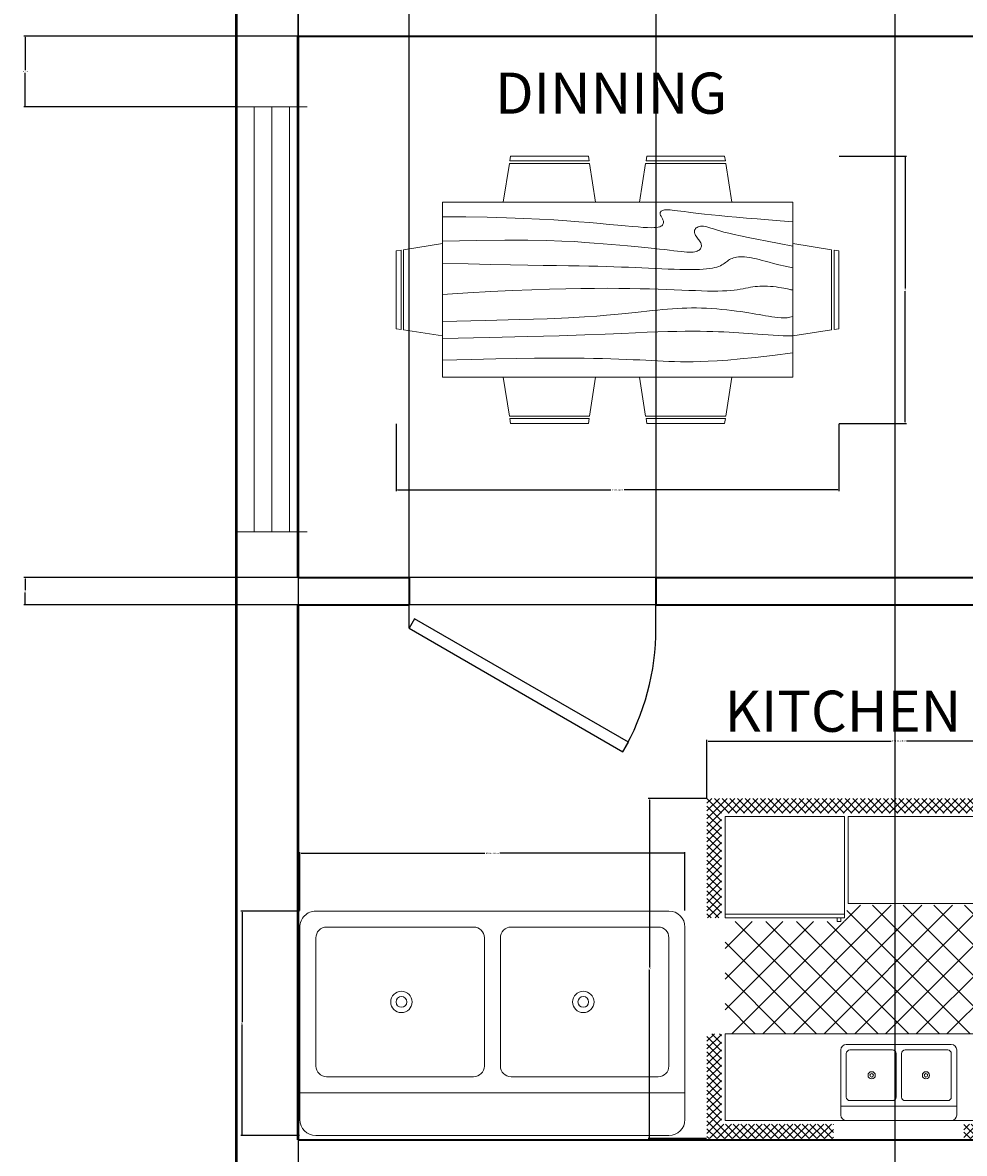
# Model space of a CAD drawing. Units: feet. Extents: x 3746 to 4170, y 1475 to 2148.
# Tile 2 of 5: x 3746 to 3884, y 1755 to 1920. Entities that reach past the tile are written whole.
import ezdxf

# ---------------------------------------------------------------- set-up
doc = ezdxf.new("R2010")
doc.units = ezdxf.units.FT
for name, color, linetype, lineweight in [('A-ANNO-DIMS', 2, 'Continuous', 18), ('A-AREA-IDEN', 7, 'Continuous', 25), ('A-FLOR-FIXT', 9, 'Continuous', 18), ('A-GLAZ', 91, 'Continuous', 18), ('DOOR', 135, 'Continuous', 25), ('FURNITURE', 43, 'Continuous', 18), ('INWER WALL', 30, 'Continuous', 35), ('OUTER WALL', 31, 'Continuous', 50)]:
    doc.layers.add(name, color=color, linetype=linetype, lineweight=lineweight)
doc.styles.get("Standard").update_dxf_attribs({"font": 'arial.ttf'})
doc.dimstyles.get("Standard").update_dxf_attribs({"dimtxt": 0.18, "dimasz": 0.18, "dimexe": 0.18, "dimexo": 0.0625, "dimgap": 0.09, "dimtad": 0, "dimtih": 1, "dimtoh": 1, "dimdec": 4, "dimzin": 0, "dimdsep": 46, "dimtxsty": 'Standard', "dimcen": 0.09, "dimadec": 0, "dimazin": 0, "dimtfac": 1, "dimtdec": 4, "dimtofl": 0, "dimtmove": 0, "dimatfit": 3, "dimfxl": 1, "dimtolj": 1, "dimtzin": 0, "dimarcsym": 0})

# ---------------------------------------------------------------- blocks, each defined once
blk = doc.blocks.new('*U3')
for p, q in [((0, 0), (0, 6)), ((40, 0), (40, 6))]:
    blk.add_line(p, q)
blk.add_lwpolyline([(0, 0), (34.64, -20), (35.52, -18.48), (0.87, 1.52)], close=True)
blk.add_arc((0, 0), 40, 330, 0)
blk = doc.blocks.new('Dining Set - 36 x 72 in.')
for p, q in [((-22.2343, 26.00059), (-23.4847, 17.99762)), ((-22.2304, 26), (-5.7608, 26)), ((-22, 27.5), (-22.1562, 26.50042)), ((-5.8416, 26.5), (-22.1534, 26.5)), ((-22, 27.5), (-6, 27.5)), ((-5.8437, 26.49966), (-6, 27.5)), ((-4.5152, 17.99762), (-5.7655, 25.99926)), ((5.7657, 26.00059), (4.5153, 17.99762)), ((5.7696, 26), (22.2392, 26)), ((6, 27.5), (5.8438, 26.50042)), ((22.1584, 26.5), (5.8466, 26.5)), ((6, 27.5), (22, 27.5)), ((22.1563, 26.49966), (22, 27.5)), ((23.4848, 17.99762), (22.2345, 25.99926)), ((36, 18), (-36, 18)), ((-36, 18), (-36, -18)), ((36, -18), (36, 18)), ((-44.0006, 8.23428), (-35.9976, 9.48474)), ((44.0006, 8.23428), (35.9976, 9.48474)), ((-45.5, 8), (-44.5004, 8.15617)), ((-45.5, 8), (-45.5, -8)), ((-44.5, -8.15843), (-44.5, 8.15338)), ((-44, 8.23041), (-44, -8.23915)), ((44, 8.23041), (44, -8.23915)), ((44.5, -8.15843), (44.5, 8.15338)), ((45.5, 8), (44.5005, 8.15617)), ((45.5, 8), (45.5, -8)), ((-44.4997, -8.15631), (-45.5, -8)), ((-35.9976, -9.48476), (-43.9993, -8.2345)), ((35.9976, -9.48476), (43.9993, -8.2345)), ((44.4997, -8.15631), (45.5, -8)), ((-36, -18), (36, -18)), ((-22.2343, -26.0006), (-23.4847, -17.99762)), ((-4.5152, -17.99762), (-5.7655, -25.99928)), ((5.7657, -26.0006), (4.5153, -17.99762)), ((23.4848, -17.99762), (22.2345, -25.99928)), ((-22.2304, -26), (-5.7608, -26)), ((-22, -27.5), (-22.1562, -26.50044)), ((-5.8416, -26.5), (-22.1534, -26.5)), ((-22, -27.5), (-6, -27.5)), ((-5.8437, -26.49967), (-6, -27.5)), ((5.7696, -26), (22.2392, -26)), ((6, -27.5), (5.8438, -26.50044)), ((22.1584, -26.5), (5.8466, -26.5)), ((6, -27.5), (22, -27.5)), ((22.1563, -26.49967), (22, -27.5))]:
    blk.add_line(p, q)
for points in [[(-36, 15), (-31.1772, 14.97754), (-26.8079, 14.91406), (-22.8538, 14.81543), (-19.276, 14.6875), (-16.0362, 14.53613), (-13.0957, 14.36718), (-10.4159, 14.18652), (-7.9583, 14), (-5.6904, 13.81315), (-3.6035, 13.63021), (-1.6954, 13.45508), (0.0365, 13.29166), (1.5945, 13.14388), (2.9811, 13.01562), (4.1988, 12.9108), (5.25, 12.83333), (6.1393, 12.78613), (6.8802, 12.76823), (7.4883, 12.77767), (7.9792, 12.8125), (8.3685, 12.87077), (8.6719, 12.95052), (8.9049, 13.0498), (9.0833, 13.16666), (9.2205, 13.29899), (9.3216, 13.44401), (9.3895, 13.59879), (9.4271, 13.76041), (9.4373, 13.92594), (9.4232, 14.09245), (9.3875, 14.257), (9.3333, 14.41666), (9.2638, 14.56917), (9.1836, 14.71484), (9.0975, 14.85465), (9.0104, 14.98958), (8.9272, 15.1206), (8.8529, 15.2487), (8.7922, 15.37483), (8.75, 15.5), (8.7305, 15.62467), (8.7344, 15.74739), (8.7617, 15.86621), (8.8125, 15.97916), (8.8867, 16.08431), (8.9844, 16.17968), (9.1055, 16.26334), (9.25, 16.33333), (9.4189, 16.38802), (9.6172, 16.42708), (9.8506, 16.45052), (10.125, 16.45833), (10.4463, 16.45052), (10.8203, 16.42708), (11.2529, 16.38802), (11.75, 16.33333), (12.3184, 16.26318), (12.9694, 16.17838), (13.7151, 16.07991), (14.5677, 15.96875), (15.5395, 15.84586), (16.6426, 15.71224), (17.8893, 15.56884), (19.2917, 15.41666), (20.859, 15.25667), (22.5879, 15.08984), (24.4721, 14.91715), (26.5052, 14.73958), (28.6809, 14.5581), (30.9929, 14.3737), (33.4347, 14.18733), (36, 14)], [(-36, 10), (-28.9766, 10.14274), (-23.1725, 10.20442), (-18.4241, 10.19775), (-14.5677, 10.13541), (-11.4399, 10.03011), (-8.877, 9.89453), (-6.7154, 9.74137), (-4.7917, 9.58333), (-2.9698, 9.43082), (-1.2246, 9.28515), (0.4415, 9.14534), (2.026, 9.01041), (3.5266, 8.87939), (4.9408, 8.7513), (6.266, 8.62516), (7.5, 8.5), (8.6411, 8.37549), (9.6914, 8.2539), (10.6538, 8.13818), (11.5312, 8.03125), (12.3267, 7.93603), (13.043, 7.85547), (13.6831, 7.79248), (14.25, 7.75), (14.7471, 7.7303), (15.1797, 7.73307), (15.5537, 7.75732), (15.875, 7.80208), (16.1494, 7.86637), (16.3828, 7.94922), (16.5811, 8.04964), (16.75, 8.16666), (16.8944, 8.29915), (17.0143, 8.44531), (17.1089, 8.60319), (17.1771, 8.77083), (17.218, 8.94629), (17.2305, 9.1276), (17.2137, 9.31282), (17.1667, 9.5), (17.0895, 9.6875), (16.987, 9.875), (16.8649, 10.0625), (16.7292, 10.25), (16.5856, 10.4375), (16.4401, 10.625), (16.2985, 10.8125), (16.1667, 11), (16.05, 11.18733), (15.9518, 11.3737), (15.8752, 11.5581), (15.8229, 11.73958), (15.798, 11.91715), (15.8034, 12.08984), (15.842, 12.25667), (15.9167, 12.41666), (16.0295, 12.56836), (16.1784, 12.70833), (16.3605, 12.83268), (16.5729, 12.9375), (16.8127, 13.01888), (17.0768, 13.07291), (17.3625, 13.0957), (17.6667, 13.08333), (17.9894, 13.03312), (18.3418, 12.94726), (18.7382, 12.82918), (19.1927, 12.68229), (19.7195, 12.51001), (20.3327, 12.31575), (21.0465, 12.10294), (21.875, 11.875), (22.8357, 11.63354), (23.959, 11.37304), (25.2786, 11.08618), (26.8282, 10.76562), (28.6414, 10.40405), (30.752, 9.99414), (33.1936, 9.52856), (36, 9)], [(-36, 5.5), (-30.7157, 5.3348), (-26.069, 5.20963), (-21.9946, 5.11767), (-18.4271, 5.05208), (-15.3009, 5.00602), (-12.5508, 4.97265), (-10.1112, 4.94515), (-7.9167, 4.91666), (-5.909, 4.88167), (-4.0586, 4.83984), (-2.3429, 4.79215), (-0.7396, 4.73958), (0.7739, 4.6831), (2.22, 4.6237), (3.6213, 4.56233), (5, 4.5), (6.373, 4.43782), (7.7344, 4.3776), (9.0723, 4.32129), (10.375, 4.27083), (11.6309, 4.22819), (12.8281, 4.19531), (13.9551, 4.17415), (15, 4.16666), (15.954, 4.17448), (16.819, 4.19791), (17.6001, 4.23698), (18.3021, 4.29166), (18.9299, 4.36198), (19.4883, 4.44791), (19.9823, 4.54948), (20.4167, 4.66666), (20.7969, 4.79899), (21.1302, 4.94401), (21.4245, 5.09879), (21.6875, 5.26041), (21.9271, 5.42594), (22.1511, 5.59245), (22.3672, 5.757), (22.5834, 5.91666), (22.8065, 6.06868), (23.0404, 6.21093), (23.2879, 6.34147), (23.5521, 6.45833), (23.8358, 6.55957), (24.142, 6.64323), (24.4735, 6.70735), (24.8334, 6.75), (25.2235, 6.76969), (25.642, 6.76692), (26.0858, 6.74267), (26.5521, 6.69791), (27.0379, 6.63362), (27.5404, 6.55078), (28.0565, 6.45036), (28.5834, 6.33333), (29.1242, 6.19987), (29.7071, 6.04687), (30.3661, 5.87044), (31.1354, 5.66666), (32.0493, 5.43164), (33.142, 5.16146), (34.4475, 4.85221), (36, 4.5)], [(-36, -1), (-30.7915, -0.6591), (-26.0195, -0.38216), (-21.6519, -0.16284), (-17.6563, 0.00521), (-14.0005, 0.12833), (-10.6523, 0.21289), (-7.5796, 0.26522), (-4.75, 0.29166), (-2.134, 0.29793), (0.2878, 0.28711), (2.5317, 0.26163), (4.6146, 0.22396), (6.5529, 0.17651), (8.3633, 0.12174), (10.0623, 0.06209), (11.6667, 0), (13.1899, -0.06201), (14.6341, -0.1211), (15.9982, -0.17432), (17.2813, -0.21875), (18.4823, -0.25147), (19.6003, -0.26953), (20.6343, -0.27002), (21.5834, -0.25), (22.4481, -0.20768), (23.2357, -0.14584), (23.9549, -0.06836), (24.6146, 0.02083), (25.2235, 0.11784), (25.7904, 0.21875), (26.3241, 0.31966), (26.8334, 0.41666), (27.3265, 0.50618), (27.8099, 0.58593), (28.2894, 0.65397), (28.7709, 0.70833), (29.2601, 0.74707), (29.763, 0.76823), (30.2855, 0.76985), (30.8334, 0.75), (31.4088, 0.70784), (31.9994, 0.64713), (32.589, 0.57275), (33.1615, 0.48958), (33.7008, 0.4025), (34.1908, 0.3164), (34.6153, 0.23616), (34.9584, 0.16666), (35.2099, 0.11165), (35.3848, 0.07031), (35.504, 0.04069), (35.5886, 0.02083), (35.6594, 0.00879), (35.7377, 0.0026), (35.8442, 0.00032), (36, 0)], [(-36, -6.5), (-27.1843, -6.31267), (-20.084, -6.1263), (-14.469, -5.9419), (-10.1094, -5.76042), (-6.7752, -5.58285), (-4.2363, -5.41016), (-2.2629, -5.24333), (-0.625, -5.08334), (0.8708, -4.93099), (2.2715, -4.78646), (3.5872, -4.64974), (4.8281, -4.52084), (6.0046, -4.39974), (7.127, -4.28646), (8.2053, -4.18099), (9.25, -4.08334), (10.2705, -3.99382), (11.2734, -3.91407), (12.2647, -3.84603), (13.25, -3.79167), (14.2354, -3.75293), (15.2266, -3.73177), (16.2295, -3.73015), (17.25, -3.75), (18.2912, -3.79248), (19.3451, -3.85547), (20.4009, -3.93604), (21.4479, -4.03125), (22.4754, -4.13819), (23.4727, -4.25391), (24.4289, -4.37549), (25.3334, -4.5), (26.1785, -4.62492), (26.9694, -4.74935), (27.7145, -4.87281), (28.4219, -4.99479), (29.1, -5.11483), (29.7572, -5.23242), (30.4016, -5.34709), (31.0417, -5.45834), (31.6837, -5.56437), (32.3262, -5.65821), (32.9658, -5.73153), (33.599, -5.77604), (34.2224, -5.78345), (34.8327, -5.74545), (35.4264, -5.65373), (36, -5.5)], [(-36, -10), (-26.4022, -9.81299), (-18.4675, -9.62891), (-11.9839, -9.45069), (-6.7396, -9.28125), (-2.5226, -9.12354), (0.8789, -8.98047), (3.6769, -8.85498), (6.0833, -8.75), (8.2767, -8.66765), (10.3021, -8.60677), (12.1712, -8.56543), (13.8958, -8.54167), (15.4876, -8.53353), (16.9583, -8.53907), (18.3197, -8.55632), (19.5834, -8.58334), (20.7616, -8.61841), (21.8685, -8.66081), (22.9188, -8.71004), (23.9271, -8.76563), (24.9081, -8.82707), (25.8763, -8.89388), (26.8465, -8.96558), (27.8334, -9.04167), (28.8474, -9.12118), (29.8828, -9.20117), (30.93, -9.27824), (31.9792, -9.34896), (33.0205, -9.40991), (34.0443, -9.45768), (35.0407, -9.48885), (36, -9.5)], [(-36, -14.5), (-30.0881, -14.33513), (-25.0332, -14.21224), (-20.7312, -14.12647), (-17.0781, -14.07292), (-13.97, -14.04671), (-11.3027, -14.04297), (-8.9724, -14.05681), (-6.875, -14.08334), (-4.9224, -14.11833), (-3.0905, -14.16016), (-1.3709, -14.20785), (0.2448, -14.26042), (1.7647, -14.3169), (3.1973, -14.3763), (4.5507, -14.43767), (5.8333, -14.5), (7.0554, -14.5621), (8.235, -14.62175), (9.3922, -14.67652), (10.5469, -14.72396), (11.7192, -14.76164), (12.929, -14.78711), (14.1965, -14.79794), (15.5417, -14.79167), (16.9933, -14.76424), (18.6152, -14.70508), (20.4804, -14.60197), (22.6615, -14.44271), (25.2312, -14.21509), (28.2624, -13.9069), (31.8277, -13.50594), (36, -13)]]:
    blk.add_lwpolyline(points)
blk = doc.blocks.new('Kitchen Layout - 7 x 8 ft')
for p, q in [((-5, 81.32), (2.68, 89)), ((-5, 83.44), (0.56, 89)), ((-5, 85.56), (-1.56, 89)), ((-5, 87.68), (-3.68, 89)), ((-1, 84.97), (-5, 88.97)), ((1.09, 85), (-2.91, 89)), ((3.21, 85), (-0.79, 89)), ((0.81, 85), (4.81, 89)), ((5.34, 85), (1.34, 89)), ((2.93, 85), (6.93, 89)), ((7.46, 85), (3.46, 89)), ((5.05, 85), (9.05, 89)), ((9.58, 85), (5.58, 89)), ((7.17, 85), (11.17, 89)), ((11.7, 85), (7.7, 89)), ((9.29, 85), (13.29, 89)), ((13.82, 85), (9.82, 89)), ((11.41, 85), (15.41, 89)), ((15.94, 85), (11.94, 89)), ((13.53, 85), (17.53, 89)), ((18.06, 85), (14.06, 89)), ((15.65, 85), (19.65, 89)), ((20.18, 85), (16.18, 89)), ((17.78, 85), (21.78, 89)), ((22.31, 85), (18.31, 89)), ((19.9, 85), (23.9, 89)), ((24.43, 85), (20.43, 89)), ((22.02, 85), (26.02, 89)), ((26.55, 85), (22.55, 89)), ((24.14, 85), (28.14, 89)), ((28.67, 85), (24.67, 89)), ((26.26, 85), (30.26, 89)), ((30.79, 85), (26.79, 89)), ((28.38, 85), (32.38, 89)), ((32.91, 85), (28.91, 89)), ((30.5, 85), (34.5, 89)), ((35.03, 85), (31.03, 89)), ((32.63, 85), (36.63, 89)), ((37.16, 85), (33.16, 89)), ((34.75, 85), (38.75, 89)), ((39.28, 85), (35.28, 89)), ((36.87, 85), (40.87, 89)), ((41.4, 85), (37.4, 89)), ((38.99, 85), (42.99, 89)), ((43.52, 85), (39.52, 89)), ((41.11, 85), (45.11, 89)), ((45.64, 85), (41.64, 89)), ((43.23, 85), (47.23, 89)), ((47.76, 85), (43.76, 89)), ((45.35, 85), (49.35, 89)), ((49.88, 85), (45.88, 89)), ((47.47, 85), (51.47, 89)), ((52, 85), (48, 89)), ((49.6, 85), (53.6, 89)), ((54.13, 85), (50.13, 89)), ((51.72, 85), (55.72, 89)), ((56.25, 85), (52.25, 89)), ((53.84, 85), (57.84, 89)), ((58.37, 85), (54.37, 89)), ((55.96, 85), (59.96, 89)), ((60.49, 85), (56.49, 89)), ((58.08, 85), (62.08, 89)), ((62.61, 85), (58.61, 89)), ((60.2, 85), (64.2, 89)), ((64.73, 85), (60.73, 89)), ((62.32, 85), (66.32, 89)), ((66.85, 85), (62.85, 89)), ((64.45, 85), (68.45, 89)), ((68.97, 85), (64.97, 89)), ((66.57, 85), (70.57, 89)), ((71.1, 85), (67.1, 89)), ((68.69, 85), (72.69, 89)), ((73.22, 85), (69.22, 89)), ((70.81, 85), (74.81, 89)), ((75.34, 85), (71.34, 89)), ((72.93, 85), (76.93, 89)), ((77.46, 85), (73.46, 89)), ((75.05, 85), (79.05, 89)), ((79.58, 85), (75.58, 89)), ((77.17, 85), (81.17, 89)), ((81.7, 85), (77.7, 89)), ((79.29, 85), (83.29, 89)), ((83.82, 85), (79.82, 89)), ((81.42, 85), (85.42, 89)), ((85.95, 85), (81.95, 89)), ((83.54, 85), (87.54, 89)), ((88.07, 85), (84.07, 89)), ((85.66, 85), (89.66, 89)), ((90.19, 85), (86.19, 89)), ((87.78, 85), (91.78, 89)), ((92.31, 85), (88.31, 89)), ((89.9, 85), (93.9, 89)), ((94.43, 85), (90.43, 89)), ((92.02, 85), (96.02, 89)), ((96.55, 85), (92.55, 89)), ((94.14, 85), (98.14, 89)), ((101, 82.67), (94.67, 89)), ((96.27, 85), (100.27, 89)), ((101, 84.79), (96.79, 89)), ((97, 83.61), (101, 87.61)), ((101, 86.92), (98.92, 89)), ((-1, 82.85), (-5, 86.85)), ((-1, 80.73), (-5, 84.73)), ((97, 81.49), (101, 85.49)), ((101, 80.55), (97, 84.55)), ((-5, 79.19), (-1, 83.19)), ((-1, 78.61), (-5, 82.61)), ((34, 84), (96, 84)), ((34, 60), (34, 84)), ((96, 84), (96, 60)), ((97, 79.37), (101, 83.37)), ((101, 78.43), (97, 82.43)), ((-5, 77.07), (-1, 81.07)), ((-1, 76.49), (-5, 80.49)), ((-5, 74.95), (-1, 78.95)), ((-1, 74.36), (-5, 78.36)), ((74, 81), (95, 81)), ((97, 77.25), (101, 81.25)), ((101, 76.31), (97, 80.31)), ((97, 75.13), (101, 79.13)), ((101, 74.19), (97, 78.19)), ((-5, 72.83), (-1, 76.83)), ((-1, 72.24), (-5, 76.24)), ((97, 73.01), (101, 77.01)), ((101, 72.07), (97, 76.07)), ((-5, 70.71), (-1, 74.71)), ((-1, 70.12), (-5, 74.12)), ((-5, 68.59), (-1, 72.59)), ((-1, 68), (-5, 72)), ((97, 70.89), (101, 74.89)), ((101, 69.95), (97, 73.95)), ((97, 68.76), (101, 72.76)), ((-5, 66.47), (-1, 70.47)), ((-1, 65.88), (-5, 69.88)), ((101, 67.82), (97, 71.82)), ((97, 66.64), (101, 70.64)), ((101, 65.7), (97, 69.7)), ((-5, 64.35), (-1, 68.35)), ((-1, 63.76), (-5, 67.76)), ((-5, 62.22), (-1, 66.22)), ((-1, 61.64), (-5, 65.64)), ((97, 64.52), (101, 68.52)), ((101, 63.58), (97, 67.58)), ((97, 62.4), (101, 66.4)), ((-5, 60.1), (-1, 64.1)), ((-1, 59.52), (-5, 63.52)), ((101, 61.46), (97, 65.46)), ((97, 60.28), (101, 64.28)), ((100.34, 60), (97, 63.34)), ((-5, 57.98), (-1, 61.98)), ((-1, 57.39), (-5, 61.39)), ((-4.86, 56), (-1, 59.86)), ((10.4, 24), (45.9, 59.5)), ((18.88, 24), (54.38, 59.5)), ((27.37, 24), (62.87, 59.5)), ((33.03, 55.11), (37.41, 59.5)), ((96, 60), (34, 60)), ((35.85, 24), (71.35, 59.5)), ((76.2, 24), (40.7, 59.5)), ((84.68, 24), (49.18, 59.5)), ((93.17, 24), (57.67, 59.5)), ((96, 29.65), (66.15, 59.5)), ((80, 60), (80, 59)), ((82, 59), (82, 60)), ((87, 59), (87, 60)), ((89, 60), (89, 59)), ((98.22, 60), (97, 61.22)), ((98.84, 60), (101, 62.16)), ((100.96, 60), (101, 60.04)), ((-1.73, 56), (-5, 59.27)), ((-3.85, 56), (-5, 57.15)), ((-2.74, 56), (-1, 57.74)), ((0, 57), (33, 57)), ((67.71, 24), (33.68, 58.04)), ((44.34, 24), (77.84, 57.5)), ((52.82, 24), (86.32, 57.5)), ((61.31, 24), (96, 58.69)), ((96, 38.14), (76.64, 57.5)), ((96, 46.63), (85.13, 57.5)), ((96, 55.11), (93.57, 57.54)), ((0, 30.57), (24.43, 55)), ((0, 39.06), (15.94, 55)), ((0, 47.54), (7.46, 55)), ((1.91, 24), (32.91, 55)), ((33.77, 24), (2.77, 55)), ((42.26, 24), (11.26, 55)), ((50.74, 24), (19.74, 55)), ((59.23, 24), (28.23, 55)), ((31, 55), (31, 56)), ((32, 55), (31, 55)), ((32, 56), (32, 55)), ((69.79, 24), (96, 50.21)), ((25.29, 24), (0, 49.29)), ((16.8, 24), (0, 40.8)), ((78.28, 24), (96, 41.72)), ((8.32, 24), (0, 32.32)), ((86.76, 24), (96, 33.24)), ((-5, 21.92), (-2.92, 24)), ((-5, 19.8), (-1, 23.8)), ((-1, 19.21), (-5, 23.21)), ((-1, 21.33), (-3.67, 24)), ((-1, 23.45), (-1.55, 24)), ((0, 24), (96, 24)), ((0, 0), (0, 24)), ((95.25, 24), (96, 24.75)), ((96, 24), (96, 0)), ((97, 22.1), (98.9, 24)), ((97, 19.97), (101, 23.97)), ((101, 19.03), (97, 23.03)), ((101, 21.16), (98.16, 24)), ((101, 23.28), (100.28, 24)), ((-5, 17.68), (-1, 21.68)), ((-1, 17.09), (-5, 21.09)), ((-5, 15.55), (-1, 19.55)), ((-1, 14.97), (-5, 18.97)), ((97, 17.85), (101, 21.85)), ((101, 16.91), (97, 20.91)), ((97, 15.73), (101, 19.73)), ((101, 14.79), (97, 18.79)), ((-5, 13.43), (-1, 17.43)), ((-1, 12.85), (-5, 16.85)), ((47.25, 6.5), (47.25, 18.5)), ((48.75, 18.5), (48.75, 6.5)), ((97, 13.61), (101, 17.61)), ((101, 12.67), (97, 16.67)), ((-5, 11.31), (-1, 15.31)), ((-1, 10.73), (-5, 14.73)), ((-5, 9.19), (-1, 13.19)), ((-1, 8.6), (-5, 12.6)), ((97, 11.49), (101, 15.49)), ((101, 10.55), (97, 14.55)), ((97, 9.37), (101, 13.37)), ((-5, 7.07), (-1, 11.07)), ((-1, 6.48), (-5, 10.48)), ((101, 8.43), (97, 12.43)), ((97, 7.25), (101, 11.25)), ((101, 6.31), (97, 10.31)), ((-5, 4.95), (-1, 8.95)), ((-1, 4.36), (-5, 8.36)), ((-5, 2.83), (-1, 6.83)), ((97, 5.12), (101, 9.12)), ((101, 4.18), (97, 8.18)), ((97, 3), (101, 7)), ((-1, 2.24), (-5, 6.24)), ((-5, 0.71), (-1, 4.71)), ((-1, 0.12), (-5, 4.12)), ((64, 4), (32, 4)), ((101, 2.06), (97, 6.06)), ((97, 0.88), (101, 4.88)), ((101, -0.06), (97, 3.94)), ((-5, -1.42), (-1, 2.58)), ((2, -5), (-5, 2)), ((-5, -3.54), (-1, 0.46)), ((96, 0), (0, 0)), ((93.24, -5), (101, 2.76)), ((95.36, -5), (101, 0.64)), ((101, -2.18), (97, 1.82)), ((-0.12, -5), (-5, -0.12)), ((-2.25, -5), (-5, -2.25)), ((-4.34, -5), (-0.34, -1)), ((-2.22, -5), (1.78, -1)), ((-0.1, -5), (3.9, -1)), ((4.12, -5), (0.12, -1)), ((2.02, -5), (6.02, -1)), ((6.24, -5), (2.24, -1)), ((4.14, -5), (8.14, -1)), ((8.36, -5), (4.36, -1)), ((6.27, -5), (10.27, -1)), ((10.48, -5), (6.48, -1)), ((8.39, -5), (12.39, -1)), ((12.6, -5), (8.6, -1)), ((10.51, -5), (14.51, -1)), ((14.73, -5), (10.73, -1)), ((12.63, -5), (16.63, -1)), ((16.85, -5), (12.85, -1)), ((14.75, -5), (18.75, -1)), ((18.97, -5), (14.97, -1)), ((16.87, -5), (20.87, -1)), ((21.09, -5), (17.09, -1)), ((18.99, -5), (22.99, -1)), ((23.21, -5), (19.21, -1)), ((21.11, -5), (25.11, -1)), ((25.33, -5), (21.33, -1)), ((23.24, -5), (27.24, -1)), ((27.45, -5), (23.45, -1)), ((25.36, -5), (29.36, -1)), ((29.57, -5), (25.57, -1)), ((27.48, -5), (30, -2.48)), ((30, -3.3), (27.7, -1)), ((30, -1.18), (29.82, -1)), ((66, -2.54), (67.54, -1)), ((66, -4.66), (69.66, -1)), ((69.88, -5), (66, -1.12)), ((67.78, -5), (71.78, -1)), ((72, -5), (68, -1)), ((69.9, -5), (73.9, -1)), ((74.12, -5), (70.12, -1)), ((72.03, -5), (76.03, -1)), ((76.24, -5), (72.24, -1)), ((74.15, -5), (78.15, -1)), ((78.36, -5), (74.36, -1)), ((76.27, -5), (80.27, -1)), ((80.49, -5), (76.49, -1)), ((78.39, -5), (82.39, -1)), ((82.61, -5), (78.61, -1)), ((80.51, -5), (84.51, -1)), ((84.73, -5), (80.73, -1)), ((82.63, -5), (86.63, -1)), ((86.85, -5), (82.85, -1)), ((84.75, -5), (88.75, -1)), ((88.97, -5), (84.97, -1)), ((86.88, -5), (90.88, -1)), ((91.09, -5), (87.09, -1)), ((89, -5), (93, -1)), ((93.21, -5), (89.21, -1)), ((91.12, -5), (95.12, -1)), ((95.34, -5), (91.34, -1)), ((97.46, -5), (93.46, -1)), ((99.58, -5), (95.58, -1)), ((101, -4.3), (97, -0.3)), ((97.48, -5), (101, -1.48)), ((-4.37, -5), (-5, -4.37)), ((29.6, -5), (30, -4.6)), ((67.76, -5), (66, -3.24)), ((99.6, -5), (101, -3.6))]:
    blk.add_line(p, q)
for points in [[(0, 56), (0, 84), (33, 84), (33, 56)], [(74, 60), (74, 84), (95, 84), (95, 60)], [(76, 58), (76, 59), (93, 59), (93, 58)]]:
    blk.add_lwpolyline(points, close=True)
for points in [[(32, 1.5), (32, 19.5)], [(33.5, 21), (62.5, 21)], [(34.5, 19.5), (46.25, 19.5)], [(49.75, 19.5), (61.5, 19.5)], [(64, 19.5), (64, 1.5)], [(33.5, 6.5), (33.5, 18.5)], [(62.5, 18.5), (62.5, 6.5)], [(46.25, 5.5), (34.5, 5.5)], [(61.5, 5.5), (49.75, 5.5)], [(62.5, 0), (33.5, 0)]]:
    blk.add_lwpolyline(points)
for centre, radius in [((80, 75), 4), ((80, 75), 3), ((80, 75), 2), ((80, 75), 1), ((89, 75), 3), ((89, 75), 2), ((89, 75), 1), ((80, 66), 3), ((89, 66), 4), ((89, 66), 3), ((80, 66), 2), ((80, 66), 1), ((89, 66), 2), ((89, 66), 1), ((40.5, 12.5), 1), ((40.5, 12.5), 0.5), ((55.5, 12.5), 1), ((55.5, 12.5), 0.5)]:
    blk.add_circle(centre, radius)
for centre, radius, start, end in [((33.5, 19.5), 1.5, 90, 180), ((34.5, 18.5), 1, 90, 180), ((46.25, 18.5), 1, 0, 90), ((49.75, 18.5), 1, 90, 180), ((61.5, 18.5), 1, 0, 90), ((62.5, 19.5), 1.5, 0, 90), ((34.5, 6.5), 1, 180, 270), ((46.25, 6.5), 1, 270, 0), ((49.75, 6.5), 1, 180, 270), ((61.5, 6.5), 1, 270, 0), ((33.5, 1.5), 1.5, 180, 270), ((62.5, 1.5), 1.5, 270, 0)]:
    blk.add_arc(centre, radius, start, end)
blk = doc.blocks.new('Sink-double - 36 in top')
for p, q in [((-18, -4), (18, -4)), ((-0.75, -18.5), (-0.75, -6.5)), ((0.75, -6.5), (0.75, -18.5))]:
    blk.add_line(p, q)
for points in [[(-16.5, 0), (16.5, 0)], [(-18, -19.5), (-18, -1.5)], [(18, -1.5), (18, -19.5)], [(-15.5, -5.5), (-1.75, -5.5)], [(1.75, -5.5), (15.5, -5.5)], [(-16.5, -18.5), (-16.5, -6.5)], [(16.5, -6.5), (16.5, -18.5)], [(-1.75, -19.5), (-15.5, -19.5)], [(15.5, -19.5), (1.75, -19.5)], [(16.5, -21), (-16.5, -21)]]:
    blk.add_lwpolyline(points)
for centre, radius in [((-8.5, -12.5), 1), ((8.5, -12.5), 1), ((-8.5, -12.5), 0.5), ((8.5, -12.5), 0.5)]:
    blk.add_circle(centre, radius)
for centre, radius, start, end in [((-16.5, -1.5), 1.5, 90, 180), ((16.5, -1.5), 1.5, 0, 90), ((-15.5, -6.5), 1, 90, 180), ((-1.75, -6.5), 1, 0, 90), ((1.75, -6.5), 1, 90, 180), ((15.5, -6.5), 1, 0, 90), ((-15.5, -18.5), 1, 180, 270), ((-1.75, -18.5), 1, 270, 0), ((1.75, -18.5), 1, 180, 270), ((15.5, -18.5), 1, 270, 0), ((-16.5, -19.5), 1.5, 180, 270), ((16.5, -19.5), 1.5, 270, 0)]:
    blk.add_arc(centre, radius, start, end)
blk = doc.blocks.new('Window - Wood Frame 36 in. Wide plan')
for p, q in [((0, 6), (0, 0)), ((36, 6), (36, 0)), ((0, 4.5), (36, 4.5)), ((0, 3), (36, 3)), ((0, 1.5), (36, 1.5))]:
    blk.add_line(p, q)
blk = doc.blocks.new('*D47')
at = {"layer": 'A-ANNO-DIMS', "color": 0, "lineweight": -2, "transparency": 16777216}
for p, q in [((3800.73, 1861.79), (3800.73, 1851.99)), ((3865.28, 1861.79), (3865.28, 1851.99)), ((3800.91, 1852.17), (3832.04, 1852.17)), ((3865.1, 1852.17), (3833.97, 1852.17))]:
    blk.add_line(p, q, dxfattribs=at)
at = {"layer": 'A-ANNO-DIMS', "color": 0, "transparency": 16777216}
for points in [[(3800.91, 1852.2), (3800.91, 1852.14), (3800.73, 1852.17)], [(3865.1, 1852.2), (3865.1, 1852.14), (3865.28, 1852.17)]]:
    blk.add_solid(points, dxfattribs=at)
at = {"layer": 'Defpoints', "color": 0, "transparency": 16777216}
for p in [(3800.73, 1861.86), (3865.28, 1861.86), (3865.28, 1852.17)]:
    blk.add_point(p, dxfattribs=at)
at = {"layer": 'A-ANNO-DIMS', "color": 0, "transparency": 16777216, "insert": (3833, 1852.17), "char_height": 0.18, "attachment_point": 5}
blk.add_mtext('\\A1;DINING SET 65', dxfattribs=at)
blk = doc.blocks.new('*D48')
at = {"layer": 'A-ANNO-DIMS', "color": 0, "lineweight": -2, "transparency": 16777216}
for p, q in [((3865.34, 1900.87), (3875.14, 1900.87)), ((3874.96, 1900.69), (3874.96, 1881.55)), ((3874.96, 1862.04), (3874.96, 1881.18)), ((3865.34, 1861.86), (3875.14, 1861.86))]:
    blk.add_line(p, q, dxfattribs=at)
at = {"layer": 'A-ANNO-DIMS', "color": 0, "transparency": 16777216}
for points in [[(3874.93, 1900.69), (3874.99, 1900.69), (3874.96, 1900.87)], [(3874.93, 1862.04), (3874.99, 1862.04), (3874.96, 1861.86)]]:
    blk.add_solid(points, dxfattribs=at)
at = {"layer": 'Defpoints', "color": 0, "transparency": 16777216}
for p in [(3865.28, 1900.87), (3874.96, 1900.87), (3865.28, 1861.86)]:
    blk.add_point(p, dxfattribs=at)
at = {"layer": 'A-ANNO-DIMS', "color": 0, "transparency": 16777216, "insert": (3874.96, 1881.36), "char_height": 0.18, "attachment_point": 5}
blk.add_mtext('\\A1;39', dxfattribs=at)
blk = doc.blocks.new('*D49')
at = {"layer": 'A-ANNO-DIMS', "color": 0, "lineweight": -2, "transparency": 16777216}
for p, q in [((3846.04, 1807.21), (3846.04, 1815.72)), ((3846.22, 1815.54), (3872.88, 1815.54)), ((3901.8, 1815.54), (3875.14, 1815.54)), ((3901.98, 1807.21), (3901.98, 1815.72))]:
    blk.add_line(p, q, dxfattribs=at)
at = {"layer": 'A-ANNO-DIMS', "color": 0, "transparency": 16777216}
for points in [[(3846.22, 1815.57), (3846.22, 1815.51), (3846.04, 1815.54)], [(3901.8, 1815.57), (3901.8, 1815.51), (3901.98, 1815.54)]]:
    blk.add_solid(points, dxfattribs=at)
at = {"layer": 'Defpoints', "color": 0, "transparency": 16777216}
for p in [(3901.98, 1815.54), (3846.04, 1807.14), (3901.98, 1807.14)]:
    blk.add_point(p, dxfattribs=at)
at = {"layer": 'A-ANNO-DIMS', "color": 0, "transparency": 16777216, "insert": (3874.01, 1815.54), "char_height": 0.18, "attachment_point": 5}
blk.add_mtext('\\A1;KITCHEN UNIT 56', dxfattribs=at)
blk = doc.blocks.new('*D50')
at = {"layer": 'A-ANNO-DIMS', "color": 0, "lineweight": -2, "transparency": 16777216}
for p, q in [((3845.98, 1807.14), (3837.47, 1807.14)), ((3837.65, 1806.96), (3837.65, 1782.52)), ((3837.65, 1757.71), (3837.65, 1782.16)), ((3845.98, 1757.53), (3837.47, 1757.53))]:
    blk.add_line(p, q, dxfattribs=at)
at = {"layer": 'A-ANNO-DIMS', "color": 0, "transparency": 16777216}
for points in [[(3837.62, 1806.96), (3837.68, 1806.96), (3837.65, 1807.14)], [(3837.62, 1757.71), (3837.68, 1757.71), (3837.65, 1757.53)]]:
    blk.add_solid(points, dxfattribs=at)
at = {"layer": 'Defpoints', "color": 0, "transparency": 16777216}
for p in [(3837.65, 1807.14), (3846.04, 1807.14), (3846.04, 1757.53)]:
    blk.add_point(p, dxfattribs=at)
at = {"layer": 'A-ANNO-DIMS', "color": 0, "transparency": 16777216, "insert": (3837.65, 1782.34), "char_height": 0.18, "attachment_point": 5}
blk.add_mtext('\\A1;50', dxfattribs=at)
blk = doc.blocks.new('*D51')
at = {"layer": 'A-ANNO-DIMS', "color": 0, "lineweight": -2, "transparency": 16777216}
for p, q in [((3786.67, 1790.8), (3786.67, 1799.34)), ((3786.85, 1799.16), (3813.65, 1799.16)), ((3842.65, 1799.16), (3815.84, 1799.16)), ((3842.83, 1790.8), (3842.83, 1799.34))]:
    blk.add_line(p, q, dxfattribs=at)
at = {"layer": 'A-ANNO-DIMS', "color": 0, "transparency": 16777216}
for points in [[(3786.85, 1799.19), (3786.85, 1799.13), (3786.67, 1799.16)], [(3842.65, 1799.19), (3842.65, 1799.13), (3842.83, 1799.16)]]:
    blk.add_solid(points, dxfattribs=at)
at = {"layer": 'Defpoints', "color": 0, "transparency": 16777216}
for p in [(3786.67, 1799.16), (3786.67, 1790.74), (3842.83, 1790.74)]:
    blk.add_point(p, dxfattribs=at)
at = {"layer": 'A-ANNO-DIMS', "color": 0, "transparency": 16777216, "insert": (3814.75, 1799.16), "char_height": 0.18, "attachment_point": 5}
blk.add_mtext('\\A1;DOUBLE SINK 56', dxfattribs=at)
blk = doc.blocks.new('*D52')
at = {"layer": 'A-ANNO-DIMS', "color": 0, "lineweight": -2, "transparency": 16777216}
for p, q in [((3786.61, 1790.74), (3778.07, 1790.74)), ((3778.25, 1790.56), (3778.25, 1774.54)), ((3778.25, 1758.16), (3778.25, 1774.18)), ((3786.61, 1757.98), (3778.07, 1757.98))]:
    blk.add_line(p, q, dxfattribs=at)
at = {"layer": 'A-ANNO-DIMS', "color": 0, "transparency": 16777216}
for points in [[(3778.22, 1790.56), (3778.28, 1790.56), (3778.25, 1790.74)], [(3778.22, 1758.16), (3778.28, 1758.16), (3778.25, 1757.98)]]:
    blk.add_solid(points, dxfattribs=at)
at = {"layer": 'Defpoints', "color": 0, "transparency": 16777216}
for p in [(3786.67, 1790.74), (3778.25, 1757.98), (3786.67, 1757.98)]:
    blk.add_point(p, dxfattribs=at)
at = {"layer": 'A-ANNO-DIMS', "color": 0, "transparency": 16777216, "insert": (3778.25, 1774.36), "char_height": 0.18, "attachment_point": 5}
blk.add_mtext('\\A1;33', dxfattribs=at)
blk = doc.blocks.new('*D63')
at = {"layer": 'A-ANNO-DIMS', "color": 0, "lineweight": -2, "transparency": 16777216}
for p, q in [((3786.43, 1970.32), (3786.43, 1474.8)), ((3873.43, 1922.32), (3873.43, 1474.8)), ((3786.61, 1474.98), (3829.71, 1474.98)), ((3873.25, 1474.98), (3830.15, 1474.98))]:
    blk.add_line(p, q, dxfattribs=at)
at = {"layer": 'A-ANNO-DIMS', "color": 0, "transparency": 16777216}
for points in [[(3786.61, 1475.01), (3786.61, 1474.95), (3786.43, 1474.98)], [(3873.25, 1475.01), (3873.25, 1474.95), (3873.43, 1474.98)]]:
    blk.add_solid(points, dxfattribs=at)
at = {"layer": 'Defpoints', "color": 0, "transparency": 16777216}
for p in [(3786.43, 1970.38), (3873.43, 1922.38), (3873.43, 1474.98)]:
    blk.add_point(p, dxfattribs=at)
at = {"layer": 'A-ANNO-DIMS', "color": 0, "transparency": 16777216, "insert": (3829.93, 1474.98), "char_height": 0.18, "attachment_point": 5}
blk.add_mtext('\\A1;87', dxfattribs=at)
blk = doc.blocks.new('*D66')
at = {"layer": 'A-ANNO-DIMS', "color": 0, "lineweight": -2, "transparency": 16777216}
for p, q in [((3786.43, 1918.45), (3786.43, 2147.69)), ((3786.61, 2147.51), (3846.15, 2147.51)), ((3906.25, 2147.51), (3846.71, 2147.51)), ((3906.43, 1918.45), (3906.43, 2147.69))]:
    blk.add_line(p, q, dxfattribs=at)
at = {"layer": 'A-ANNO-DIMS', "color": 0, "transparency": 16777216}
for points in [[(3786.61, 2147.54), (3786.61, 2147.48), (3786.43, 2147.51)], [(3906.25, 2147.54), (3906.25, 2147.48), (3906.43, 2147.51)]]:
    blk.add_solid(points, dxfattribs=at)
at = {"layer": 'Defpoints', "color": 0, "transparency": 16777216}
for p in [(3906.43, 2147.51), (3786.43, 1918.38), (3906.43, 1918.38)]:
    blk.add_point(p, dxfattribs=at)
at = {"layer": 'A-ANNO-DIMS', "color": 0, "transparency": 16777216, "insert": (3846.43, 2147.51), "char_height": 0.18, "attachment_point": 5}
blk.add_mtext('\\A1;120', dxfattribs=at)
blk = doc.blocks.new('*D68')
at = {"layer": 'A-ANNO-DIMS', "color": 0, "lineweight": -2, "transparency": 16777216}
for p, q in [((3786.43, 1757.32), (3786.43, 1474.8)), ((3902.43, 1757.32), (3902.43, 1474.8)), ((3786.61, 1474.98), (3844.15, 1474.98)), ((3902.25, 1474.98), (3844.71, 1474.98))]:
    blk.add_line(p, q, dxfattribs=at)
at = {"layer": 'A-ANNO-DIMS', "color": 0, "transparency": 16777216}
for points in [[(3786.61, 1475.01), (3786.61, 1474.95), (3786.43, 1474.98)], [(3902.25, 1475.01), (3902.25, 1474.95), (3902.43, 1474.98)]]:
    blk.add_solid(points, dxfattribs=at)
at = {"layer": 'Defpoints', "color": 0, "transparency": 16777216}
for p in [(3786.43, 1757.38), (3902.43, 1757.38), (3902.43, 1474.98)]:
    blk.add_point(p, dxfattribs=at)
at = {"layer": 'A-ANNO-DIMS', "color": 0, "transparency": 16777216, "insert": (3844.43, 1474.98), "char_height": 0.18, "attachment_point": 5}
blk.add_mtext('\\A1;116', dxfattribs=at)
blk = doc.blocks.new('*D69')
at = {"layer": 'A-ANNO-DIMS', "color": 0, "lineweight": -2, "transparency": 16777216}
for p, q in [((3802.61, 1835.45), (3802.61, 2147.69)), ((3802.79, 2147.51), (3820.39, 2147.51)), ((3838.43, 2147.51), (3820.83, 2147.51)), ((3838.61, 1835.45), (3838.61, 2147.69))]:
    blk.add_line(p, q, dxfattribs=at)
at = {"layer": 'A-ANNO-DIMS', "color": 0, "transparency": 16777216}
for points in [[(3802.79, 2147.54), (3802.79, 2147.48), (3802.61, 2147.51)], [(3838.43, 2147.54), (3838.43, 2147.48), (3838.61, 2147.51)]]:
    blk.add_solid(points, dxfattribs=at)
at = {"layer": 'Defpoints', "color": 0, "transparency": 16777216}
for p in [(3838.61, 2147.51), (3802.61, 1835.38), (3838.61, 1835.38)]:
    blk.add_point(p, dxfattribs=at)
at = {"layer": 'A-ANNO-DIMS', "color": 0, "transparency": 16777216, "insert": (3820.61, 2147.51), "char_height": 0.18, "attachment_point": 5}
blk.add_mtext('\\A1;36', dxfattribs=at)
blk = doc.blocks.new('*D70')
at = {"layer": 'A-ANNO-DIMS', "color": 0, "lineweight": -2, "transparency": 16777216}
for p, q in [((3786.43, 1839.45), (3786.43, 2147.69)), ((3786.61, 2147.51), (3794.13, 2147.51)), ((3802.43, 2147.51), (3794.9, 2147.51)), ((3802.61, 1839.45), (3802.61, 2147.69))]:
    blk.add_line(p, q, dxfattribs=at)
at = {"layer": 'A-ANNO-DIMS', "color": 0, "transparency": 16777216}
for points in [[(3786.61, 2147.54), (3786.61, 2147.48), (3786.43, 2147.51)], [(3802.43, 2147.54), (3802.43, 2147.48), (3802.61, 2147.51)]]:
    blk.add_solid(points, dxfattribs=at)
at = {"layer": 'Defpoints', "color": 0, "transparency": 16777216}
for p in [(3802.61, 2147.51), (3786.43, 1839.38), (3802.61, 1839.38)]:
    blk.add_point(p, dxfattribs=at)
at = {"layer": 'A-ANNO-DIMS', "color": 0, "transparency": 16777216, "insert": (3794.52, 2147.51), "char_height": 0.18, "attachment_point": 5}
blk.add_mtext('\\A1;16.18', dxfattribs=at)
blk = doc.blocks.new('*D71')
at = {"layer": 'A-ANNO-DIMS', "color": 0, "lineweight": -2, "transparency": 16777216}
for p, q in [((3838.545248, 1839.38283), (3746.4489, 1839.38283)), ((3746.6289, 1839.20283), (3746.6289, 1837.56283)), ((3746.6289, 1835.56283), (3746.6289, 1837.20283)), ((3838.545248, 1835.38283), (3746.4489, 1835.38283))]:
    blk.add_line(p, q, dxfattribs=at)
at = {"layer": 'A-ANNO-DIMS', "color": 0, "transparency": 16777216}
for points in [[(3746.5989, 1839.20283), (3746.6589, 1839.20283), (3746.6289, 1839.38283)], [(3746.5989, 1835.56283), (3746.6589, 1835.56283), (3746.6289, 1835.38283)]]:
    blk.add_solid(points, dxfattribs=at)
at = {"layer": 'Defpoints', "color": 0, "transparency": 16777216}
for p in [(3838.607748, 1839.38283), (3746.6289, 1835.38283), (3838.607748, 1835.38283)]:
    blk.add_point(p, dxfattribs=at)
at = {"layer": 'A-ANNO-DIMS', "color": 0, "transparency": 16777216, "insert": (3746.6289, 1837.38283), "char_height": 0.18, "attachment_point": 5}
blk.add_mtext('\\A1;4', dxfattribs=at)
blk = doc.blocks.new('*D87')
at = {"layer": 'A-ANNO-DIMS', "color": 0, "lineweight": -2, "transparency": 16777216}
for p, q in [((3786.37, 1918.38), (3746.45, 1918.38)), ((3746.63, 1918.2), (3746.63, 1913.4)), ((3746.63, 1908.22), (3746.63, 1913.03)), ((3777.37, 1908.04), (3746.45, 1908.04))]:
    blk.add_line(p, q, dxfattribs=at)
at = {"layer": 'A-ANNO-DIMS', "color": 0, "transparency": 16777216}
for points in [[(3746.6, 1918.2), (3746.66, 1918.2), (3746.63, 1918.38)], [(3746.6, 1908.22), (3746.66, 1908.22), (3746.63, 1908.04)]]:
    blk.add_solid(points, dxfattribs=at)
at = {"layer": 'Defpoints', "color": 0, "transparency": 16777216}
for p in [(3786.43, 1918.38), (3746.63, 1908.04), (3777.43, 1908.04)]:
    blk.add_point(p, dxfattribs=at)
at = {"layer": 'A-ANNO-DIMS', "color": 0, "transparency": 16777216, "insert": (3746.63, 1913.21), "char_height": 0.18, "attachment_point": 5}
blk.add_mtext('\\A1;10.339', dxfattribs=at)

msp = doc.modelspace()

# ---------------------------------------------------------------- linework, layer by layer
at = {"layer": 'INWER WALL'}
for p, q in [((3786.4289, 1918.3828), (3906.4289, 1918.3828)), ((3786.4289, 1839.3828), (3802.6077, 1839.3828)), ((3802.6077, 1839.3828), (3802.6077, 1835.3828)), ((3838.6077, 1839.3828), (3838.6077, 1835.3828)), ((3838.6077, 1839.3828), (3906.4289, 1839.3828)), ((3786.4289, 1835.3828), (3802.6077, 1835.3828)), ((3838.6077, 1835.3828), (3902.4289, 1835.3828)), ((3786.4289, 1757.3828), (3902.4289, 1757.3828))]:
    msp.add_line(p, q, dxfattribs=at)
at = {"layer": 'OUTER WALL'}
for p, q in [((3786.4289, 1839.3828), (3786.4289, 1918.3828)), ((3786.4289, 1757.3828), (3786.4289, 1835.3828))]:
    msp.add_line(p, q, dxfattribs=at)
msp.add_lwpolyline([(3948.7526, 1635.3828), (3777.4289, 1635.3828), (3777.4289, 2115.3828), (4137.4289, 2115.3828), (4137.4289, 1635.3828), (4068.7526, 1635.3828)], dxfattribs=at)

# ---------------------------------------------------------------- block references
at = {"layer": 'A-FLOR-FIXT', "xscale": 0.5277695624753019, "yscale": 0.5277695624753019, "zscale": 0.5277695624753019}
msp.add_blockref('Kitchen Layout - 7 x 8 ft', (3848.6802, 1760.1735), dxfattribs=at)
at = {"layer": 'A-FLOR-FIXT', "xscale": 1.559823421486259, "yscale": 1.559823421486259, "zscale": 1.559823421486259, "rotation": 180}
msp.add_blockref('Sink-double - 36 in top', (3814.7494, 1757.9799), dxfattribs=at)
at = {"layer": 'A-GLAZ', "xscale": 1.721338572628536, "yscale": 1.721338572628536, "zscale": 1.721338572628536, "rotation": 90}
msp.add_blockref('Window - Wood Frame 36 in. Wide plan', (3787.7569, 1846.0761), dxfattribs=at)
at = {"layer": 'DOOR', "xscale": 0.9000000000000054, "yscale": 0.9000000000000054, "zscale": 0.9000000000000054}
msp.add_blockref('*U3', (3802.6077, 1831.9828), dxfattribs=at)
at = {"layer": 'FURNITURE', "xscale": 0.7093758322016473, "yscale": 0.7093758322016473, "zscale": 0.7093758322016473}
msp.add_blockref('Dining Set - 36 x 72 in.', (3833.0049, 1881.3635), dxfattribs=at)

# ---------------------------------------------------------------- texts
at = {"layer": 'A-AREA-IDEN', "char_height": 6, "attachment_point": 1}
for s, insert in [('DINNING', (3815.1379, 1913.0446)), ('KITCHEN', (3848.6112, 1822.8838))]:
    msp.add_mtext_dynamic_manual_height_columns(s, width=45.721785, gutter_width=12.5, heights=[0], dxfattribs=dict(at, insert=insert))

# ---------------------------------------------------------------- dimensions: what is measured, and where the dimension line sits
at = {"layer": 'A-ANNO-DIMS'}
for base, p1, p2, override, picture, middle in [((3906.4289, 2147.5109), (3786.4289, 1918.3828), (3906.4289, 1918.3828), {"dimdec": 0, "dimlfac": 1, "dimrnd": 0, "dimzin": 0, "dimdsep": 46, "dimlunit": 2}, '*D66', (3846.4289, 2147.5109)), ((3802.6077, 2147.5109), (3786.4289, 1839.3828), (3802.6077, 1839.3828), {"dimdec": 2, "dimlfac": 1, "dimrnd": 0, "dimzin": 0, "dimdsep": 46, "dimlunit": 2}, '*D70', (3794.5183, 2147.5109)), ((3838.6077, 2147.5109), (3802.6077, 1835.3828), (3838.6077, 1835.3828), {"dimdec": 0, "dimlfac": 1, "dimrnd": 0, "dimzin": 0, "dimdsep": 46, "dimlunit": 2}, '*D69', (3820.6077, 2147.5109)), ((3873.4289, 1474.98), (3786.4289, 1970.3828), (3873.4289, 1922.3828), {"dimdec": 0, "dimlfac": 1, "dimrnd": 0, "dimzin": 0, "dimdsep": 46, "dimlunit": 2}, '*D63', (3829.9289, 1474.98)), ((3902.4289, 1474.98), (3786.4289, 1757.3828), (3902.4289, 1757.3828), {"dimdec": 0, "dimlfac": 1, "dimrnd": 0, "dimzin": 0, "dimdsep": 46, "dimlunit": 2}, '*D68', (3844.4289, 1474.98))]:
    dim = msp.add_linear_dim(base=base, p1=p1, p2=p2, dimstyle='Standard', override=override, dxfattribs=at)
    dim.commit()
    dim.dimension.update_dxf_attribs({"geometry": picture, "text_midpoint": middle})
for base, p1, p2, angle, override, picture, middle in [((3746.6289, 1908.04431), (3786.4289, 1918.38283), (3777.4289, 1908.04431), 90, {"dimdec": 3, "dimlfac": 1, "dimrnd": 0, "dimzin": 0, "dimdsep": 46, "dimlunit": 2}, '*D87', (3746.6289, 1913.21357)), ((3874.9645, 1900.8713), (3865.2815, 1861.8556), (3865.2815, 1900.8713), 90, {"dimdec": 0, "dimlfac": 1, "dimrnd": 0, "dimzin": 0, "dimdsep": 46, "dimlunit": 2}, '*D48', (3874.9645, 1881.3635)), ((3746.6289, 1835.3828), (3838.6077, 1839.3828), (3838.6077, 1835.3828), 90, {"dimdec": 0, "dimlfac": 1, "dimrnd": 0, "dimzin": 0, "dimdsep": 46, "dimlunit": 2}, '*D71', (3746.6289, 1837.3828)), ((3837.6498, 1807.145), (3846.0414, 1757.5346), (3846.0414, 1807.145), 90, {"dimdec": 0, "dimlfac": 1, "dimrnd": 0, "dimzin": 0, "dimdsep": 46, "dimlunit": 2}, '*D50', (3837.6498, 1782.3398)), ((3778.2496, 1757.9799), (3786.6726, 1790.7362), (3786.6726, 1757.9799), 270, {"dimdec": 0, "dimlfac": 1, "dimrnd": 0, "dimzin": 0, "dimdsep": 46, "dimlunit": 2}, '*D52', (3778.2496, 1774.358))]:
    dim = msp.add_linear_dim(base=base, p1=p1, p2=p2, angle=angle, dimstyle='Standard', override=override, dxfattribs=at)
    dim.commit()
    dim.dimension.update_dxf_attribs({"geometry": picture, "text_midpoint": middle})
for base, p1, p2, text, picture, middle in [((3865.2815, 1852.1727), (3800.7283, 1861.8556), (3865.2815, 1861.8556), 'DINING SET <>', '*D47', (3833.0049, 1852.1727)), ((3901.985, 1815.5365), (3846.0414, 1807.145), (3901.985, 1807.145), 'KITCHEN UNIT <>', '*D49', (3874.0132, 1815.5365))]:
    dim = msp.add_linear_dim(base=base, p1=p1, p2=p2, text=text, dimstyle='Standard', override={"dimdec": 0, "dimlfac": 1, "dimrnd": 0, "dimzin": 0, "dimdsep": 46, "dimlunit": 2}, dxfattribs=at)
    dim.commit()
    dim.dimension.update_dxf_attribs({"geometry": picture, "text_midpoint": middle})
dim = msp.add_linear_dim(base=(3786.6726, 1799.1592), p1=(3842.8263, 1790.7362), p2=(3786.6726, 1790.7362), angle=180, text='DOUBLE SINK <>', dimstyle='Standard', override={"dimdec": 0, "dimlfac": 1, "dimrnd": 0, "dimzin": 0, "dimdsep": 46, "dimlunit": 2}, dxfattribs=at)
dim.commit()
dim.dimension.update_dxf_attribs({"geometry": '*D51', "text_midpoint": (3814.7494, 1799.1592)})

doc.saveas('drawing.dxf')
